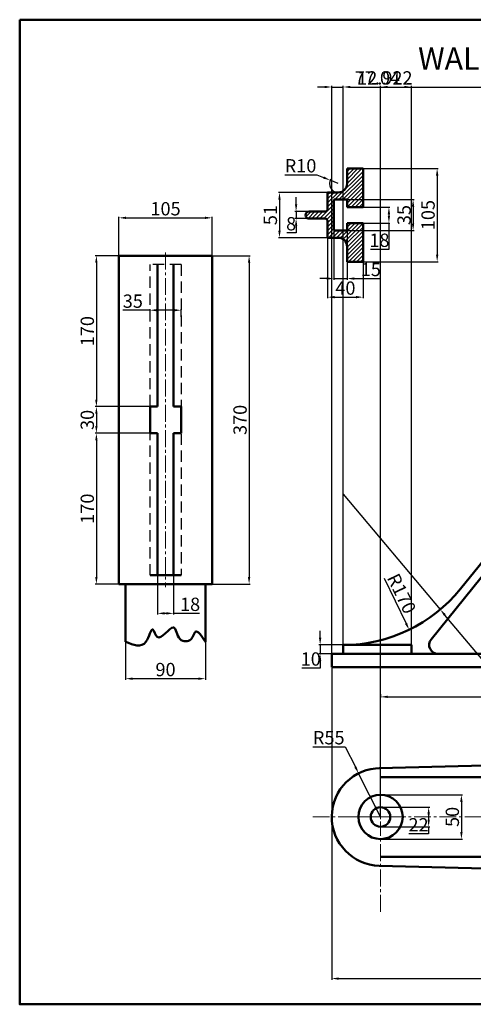
# Model space of a CAD drawing. Units: millimetres. Extents: x -60 to 1204, y -103 to 1006.
# Tile 1 of 4: x -60 to 452, y -103 to 1006. Entities that reach past the tile are written whole.
import ezdxf

# ---------------------------------------------------------------- set-up
doc = ezdxf.new("R2010")
doc.units = ezdxf.units.MM
doc.linetypes.add('CENTER2', pattern=[28.575, 19.05, -3.175, 3.175, -3.175])
doc.linetypes.add('DASHED', pattern=[19.05, 12.7, -6.35])
for name, color, linetype, lineweight in [('M-CNTR', 1, 'CENTER2', 18), ('M-DIMS', 2, 'Continuous', 25), ('M-HATC', 8, 'Continuous', 18), ('M-HIDN', 4, 'DASHED', 25), ('M-OUTL', 7, 'Continuous', 50), ('M-TEXT', 7, 'Continuous', 25), ('M-TTLB', 7, 'Continuous', 50)]:
    doc.layers.add(name, color=color, linetype=linetype, lineweight=lineweight)
doc.styles.get("Standard").update_dxf_attribs({"font": 'arial.ttf'})
doc.dimstyles.new('ISO-25', dxfattribs={"dimtxt": 15, "dimasz": 8, "dimexe": 1.25, "dimexo": 0.625, "dimtad": 1, "dimtoh": 1, "dimdec": 0, "dimtxsty": 'Standard', "dimcen": 2.5, "dimadec": 0, "dimazin": 0, "dimtfac": 1, "dimtdec": 0, "dimtmove": 0, "dimatfit": 3, "dimfxl": 1, "dimarcsym": 0})

# ---------------------------------------------------------------- blocks, each defined once
blk = doc.blocks.new('*U1')
at = {"layer": 'M-CNTR', "color": 0, "transparency": 16777216}
for p, q in [((0, 5), (0, 235.1)), ((-28.5, 0), (-5, 0)), ((5, 0), (28.5, 0)), ((0, -106.9), (0, -5))]:
    blk.add_line(p, q, dxfattribs=at)
at = {"layer": 'M-CNTR', "color": 0, "linetype": 'Continuous', "transparency": 16777216}
for p, q in [((-2.5, 0), (2.5, 0)), ((0, -2.5), (0, 2.5))]:
    blk.add_line(p, q, dxfattribs=at)
blk = doc.blocks.new('*U5')
at = {"layer": 'M-CNTR', "color": 0, "transparency": 16777216}
blk.add_line((0, 188.5), (0, -188.5), dxfattribs=at)
blk = doc.blocks.new('*D6')
at = {"layer": 'Defpoints', "color": 0, "transparency": 16777216}
for p in [(157.5, 740.2), (157.5, 370.2), (199.3, 370.2)]:
    blk.add_point(p, dxfattribs=at)
at = {"layer": 'M-DIMS', "color": 0, "lineweight": -2, "transparency": 16777216}
for p, q in [((158.1, 740.2), (200.5, 740.2)), ((199.3, 732.2), (199.3, 378.2)), ((158.1, 370.2), (200.5, 370.2))]:
    blk.add_line(p, q, dxfattribs=at)
at = {"layer": 'M-DIMS', "color": 0, "transparency": 16777216}
for points in [[(197.9, 732.2), (200.6, 732.2), (199.3, 740.2)], [(197.9, 378.2), (200.6, 378.2), (199.3, 370.2)]]:
    blk.add_solid(points, dxfattribs=at)
at = {"layer": 'M-DIMS', "color": 0, "transparency": 16777216, "insert": (191, 555.2), "char_height": 15, "attachment_point": 5, "rotation": 90}
blk.add_mtext('370', dxfattribs=at)
blk = doc.blocks.new('*D7')
at = {"layer": 'Defpoints', "color": 0, "transparency": 16777216}
for p in [(157.5, 782.9), (52.5, 740.2), (157.5, 740.2)]:
    blk.add_point(p, dxfattribs=at)
at = {"layer": 'M-DIMS', "color": 0, "lineweight": -2, "transparency": 16777216}
for p, q in [((52.5, 740.8), (52.5, 784.2)), ((60.5, 782.9), (149.5, 782.9)), ((157.5, 740.8), (157.5, 784.2))]:
    blk.add_line(p, q, dxfattribs=at)
at = {"layer": 'M-DIMS', "color": 0, "transparency": 16777216}
for points in [[(60.5, 784.2), (60.5, 781.6), (52.5, 782.9)], [(149.5, 784.2), (149.5, 781.6), (157.5, 782.9)]]:
    blk.add_solid(points, dxfattribs=at)
at = {"layer": 'M-DIMS', "color": 0, "transparency": 16777216, "insert": (105, 791.2), "char_height": 15, "attachment_point": 5}
blk.add_mtext('105', dxfattribs=at)
blk = doc.blocks.new('*D8')
at = {"layer": 'Defpoints', "color": 0, "transparency": 16777216}
for p in [(87.5, 570.2), (27, 540.2), (87.5, 540.2)]:
    blk.add_point(p, dxfattribs=at)
at = {"layer": 'M-DIMS', "color": 0, "lineweight": -2, "transparency": 16777216}
for p, q in [((86.9, 570.2), (25.7, 570.2)), ((27, 562.2), (27, 548.2)), ((86.9, 540.2), (25.7, 540.2))]:
    blk.add_line(p, q, dxfattribs=at)
at = {"layer": 'M-DIMS', "color": 0, "transparency": 16777216}
for points in [[(25.7, 562.2), (28.3, 562.2), (27, 570.2)], [(25.7, 548.2), (28.3, 548.2), (27, 540.2)]]:
    blk.add_solid(points, dxfattribs=at)
at = {"layer": 'M-DIMS', "color": 0, "transparency": 16777216, "insert": (18.7, 555.2), "char_height": 15, "attachment_point": 5, "rotation": 90}
blk.add_mtext('30', dxfattribs=at)
blk = doc.blocks.new('*D9')
at = {"layer": 'Defpoints', "color": 0, "transparency": 16777216}
for p in [(52.5, 740.2), (27, 570.2), (52.5, 570.2)]:
    blk.add_point(p, dxfattribs=at)
at = {"layer": 'M-DIMS', "color": 0, "lineweight": -2, "transparency": 16777216}
for p, q in [((51.9, 740.2), (25.7, 740.2)), ((27, 732.2), (27, 578.2)), ((51.9, 570.2), (25.7, 570.2))]:
    blk.add_line(p, q, dxfattribs=at)
at = {"layer": 'M-DIMS', "color": 0, "transparency": 16777216}
for points in [[(25.6, 732.2), (28.3, 732.2), (27, 740.2)], [(25.6, 578.2), (28.3, 578.2), (27, 570.2)]]:
    blk.add_solid(points, dxfattribs=at)
at = {"layer": 'M-DIMS', "color": 0, "transparency": 16777216, "insert": (18.7, 655.2), "char_height": 15, "attachment_point": 5, "rotation": 90}
blk.add_mtext('170', dxfattribs=at)
blk = doc.blocks.new('*D10')
at = {"layer": 'Defpoints', "color": 0, "transparency": 16777216}
for p in [(52.5, 540.2), (27, 370.2), (52.5, 370.2)]:
    blk.add_point(p, dxfattribs=at)
at = {"layer": 'M-DIMS', "color": 0, "lineweight": -2, "transparency": 16777216}
for p, q in [((51.9, 540.2), (25.7, 540.2)), ((27, 532.2), (27, 378.2)), ((51.9, 370.2), (25.7, 370.2))]:
    blk.add_line(p, q, dxfattribs=at)
at = {"layer": 'M-DIMS', "color": 0, "transparency": 16777216}
for points in [[(25.7, 532.2), (28.3, 532.2), (27, 540.2)], [(25.7, 378.2), (28.3, 378.2), (27, 370.2)]]:
    blk.add_solid(points, dxfattribs=at)
at = {"layer": 'M-DIMS', "color": 0, "transparency": 16777216, "insert": (18.7, 455.2), "char_height": 15, "attachment_point": 5, "rotation": 90}
blk.add_mtext('170', dxfattribs=at)
blk = doc.blocks.new('*D11')
at = {"layer": 'Defpoints', "color": 0, "transparency": 16777216}
for p in [(60, 321.7), (150, 321.7), (150, 263.7)]:
    blk.add_point(p, dxfattribs=at)
at = {"layer": 'M-DIMS', "color": 0, "lineweight": -2, "transparency": 16777216}
for p, q in [((60, 321.1), (60, 262.4)), ((150, 321.1), (150, 262.4)), ((68, 263.7), (142, 263.7))]:
    blk.add_line(p, q, dxfattribs=at)
at = {"layer": 'M-DIMS', "color": 0, "transparency": 16777216}
for points in [[(68, 265), (68, 262.3), (60, 263.7)], [(142, 265), (142, 262.3), (150, 263.7)]]:
    blk.add_solid(points, dxfattribs=at)
at = {"layer": 'M-DIMS', "color": 0, "transparency": 16777216, "insert": (105, 272), "char_height": 15, "attachment_point": 5}
blk.add_mtext('90', dxfattribs=at)
blk = doc.blocks.new('*D12')
at = {"layer": 'Defpoints', "color": 0, "transparency": 16777216}
for p in [(96, 380.2), (114, 380.2), (114, 337.3)]:
    blk.add_point(p, dxfattribs=at)
at = {"layer": 'M-DIMS', "color": 0, "lineweight": -2, "transparency": 16777216}
for p, q in [((96, 379.5), (96, 336)), ((114, 379.5), (114, 336)), ((104, 337.3), (106, 337.3)), ((114, 337.3), (143.4, 337.3))]:
    blk.add_line(p, q, dxfattribs=at)
at = {"layer": 'M-DIMS', "color": 0, "transparency": 16777216}
for points in [[(104, 338.6), (104, 335.9), (96, 337.3)], [(106, 338.6), (106, 335.9), (114, 337.3)]]:
    blk.add_solid(points, dxfattribs=at)
at = {"layer": 'M-DIMS', "color": 0, "transparency": 16777216, "insert": (132.7, 345.5), "char_height": 15, "attachment_point": 5}
blk.add_mtext('18', dxfattribs=at)
blk = doc.blocks.new('*D13')
at = {"layer": 'Defpoints', "color": 0, "transparency": 16777216}
for p in [(122.5, 678.8), (87.5, 670.6), (122.5, 670.6)]:
    blk.add_point(p, dxfattribs=at)
at = {"layer": 'M-DIMS', "color": 0, "lineweight": -2, "transparency": 16777216}
for p, q in [((87.5, 678.8), (56.7, 678.8)), ((87.5, 671.2), (87.5, 680.1)), ((114.5, 678.8), (95.5, 678.8)), ((122.5, 671.2), (122.5, 680.1))]:
    blk.add_line(p, q, dxfattribs=at)
at = {"layer": 'M-DIMS', "color": 0, "transparency": 16777216}
for points in [[(95.5, 680.2), (95.5, 677.5), (87.5, 678.8)], [(114.5, 680.2), (114.5, 677.5), (122.5, 678.8)]]:
    blk.add_solid(points, dxfattribs=at)
at = {"layer": 'M-DIMS', "color": 0, "transparency": 16777216, "insert": (68.1, 687.1), "char_height": 15, "attachment_point": 5}
blk.add_mtext('35', dxfattribs=at)
blk = doc.blocks.new('*D14')
at = {"layer": 'Defpoints', "color": 0, "transparency": 16777216}
for p in [(327.9, 795), (327.9, 777), (357, 777)]:
    blk.add_point(p, dxfattribs=at)
at = {"layer": 'M-DIMS', "color": 0, "lineweight": -2, "transparency": 16777216}
for p, q in [((328.5, 795), (358.2, 795)), ((328.5, 777), (358.2, 777)), ((357, 787), (357, 785)), ((357, 777), (357, 747.4)), ((357, 747.4), (336.3, 747.4))]:
    blk.add_line(p, q, dxfattribs=at)
at = {"layer": 'M-DIMS', "color": 0, "transparency": 16777216}
for points in [[(355.7, 787), (358.3, 787), (357, 795)], [(355.7, 785), (358.3, 785), (357, 777)]]:
    blk.add_solid(points, dxfattribs=at)
at = {"layer": 'M-DIMS', "color": 0, "transparency": 16777216, "insert": (346.3, 755.7), "char_height": 15, "attachment_point": 5}
blk.add_mtext('18', dxfattribs=at)
blk = doc.blocks.new('*D15')
at = {"layer": 'Defpoints', "color": 0, "transparency": 16777216}
for p in [(309.9, 803.5), (309.9, 768.5), (384.3, 768.5)]:
    blk.add_point(p, dxfattribs=at)
at = {"layer": 'M-DIMS', "color": 0, "lineweight": -2, "transparency": 16777216}
for p, q in [((310.5, 803.5), (385.5, 803.5)), ((384.3, 795.5), (384.3, 776.5)), ((310.5, 768.5), (385.5, 768.5))]:
    blk.add_line(p, q, dxfattribs=at)
at = {"layer": 'M-DIMS', "color": 0, "transparency": 16777216}
for points in [[(382.9, 795.5), (385.6, 795.5), (384.3, 803.5)], [(382.9, 776.5), (385.6, 776.5), (384.3, 768.5)]]:
    blk.add_solid(points, dxfattribs=at)
at = {"layer": 'M-DIMS', "color": 0, "transparency": 16777216, "insert": (376, 786), "char_height": 15, "attachment_point": 5, "rotation": 90}
blk.add_mtext('35', dxfattribs=at)
blk = doc.blocks.new('*D16')
at = {"layer": 'Defpoints', "color": 0, "transparency": 16777216}
for p in [(327.9, 838.5), (327.9, 733.5), (411.4, 733.5)]:
    blk.add_point(p, dxfattribs=at)
at = {"layer": 'M-DIMS', "color": 0, "lineweight": -2, "transparency": 16777216}
for p, q in [((328.5, 838.5), (412.7, 838.5)), ((411.4, 830.5), (411.4, 741.5)), ((328.5, 733.5), (412.7, 733.5))]:
    blk.add_line(p, q, dxfattribs=at)
at = {"layer": 'M-DIMS', "color": 0, "transparency": 16777216}
for points in [[(410.1, 830.5), (412.8, 830.5), (411.4, 838.5)], [(410.1, 741.5), (412.8, 741.5), (411.4, 733.5)]]:
    blk.add_solid(points, dxfattribs=at)
at = {"layer": 'M-DIMS', "color": 0, "transparency": 16777216, "insert": (403.1, 786), "char_height": 15, "attachment_point": 5, "rotation": 90}
blk.add_mtext('105', dxfattribs=at)
blk = doc.blocks.new('*D17')
at = {"layer": 'Defpoints', "color": 0, "transparency": 16777216}
for p in [(293.9, 811.5), (233.5, 760.5), (293.9, 760.5)]:
    blk.add_point(p, dxfattribs=at)
at = {"layer": 'M-DIMS', "color": 0, "lineweight": -2, "transparency": 16777216}
for p, q in [((293.2, 811.5), (232.3, 811.5)), ((233.5, 803.5), (233.5, 768.5)), ((293.2, 760.5), (232.3, 760.5))]:
    blk.add_line(p, q, dxfattribs=at)
at = {"layer": 'M-DIMS', "color": 0, "transparency": 16777216}
for points in [[(232.2, 803.5), (234.9, 803.5), (233.5, 811.5)], [(232.2, 768.5), (234.9, 768.5), (233.5, 760.5)]]:
    blk.add_solid(points, dxfattribs=at)
at = {"layer": 'M-DIMS', "color": 0, "transparency": 16777216, "insert": (225.2, 786), "char_height": 15, "attachment_point": 5, "rotation": 90}
blk.add_mtext('51', dxfattribs=at)
blk = doc.blocks.new('*D18')
at = {"layer": 'Defpoints', "color": 0, "transparency": 16777216}
for p in [(275.9, 790), (252.3, 782), (275.9, 782)]:
    blk.add_point(p, dxfattribs=at)
at = {"layer": 'M-DIMS', "color": 0, "lineweight": -2, "transparency": 16777216}
for p, q in [((252.3, 798), (252.3, 806)), ((275.2, 790), (251, 790)), ((252.3, 790), (252.3, 782)), ((275.2, 782), (251, 782)), ((252.3, 766), (241.8, 766)), ((252.3, 774), (252.3, 766))]:
    blk.add_line(p, q, dxfattribs=at)
at = {"layer": 'M-DIMS', "color": 0, "transparency": 16777216}
for points in [[(251, 798), (253.6, 798), (252.3, 790)], [(251, 774), (253.6, 774), (252.3, 782)]]:
    blk.add_solid(points, dxfattribs=at)
at = {"layer": 'M-DIMS', "color": 0, "transparency": 16777216, "insert": (246.7, 774.3), "char_height": 15, "attachment_point": 5}
blk.add_mtext('8', dxfattribs=at)
blk = doc.blocks.new('*D19')
at = {"layer": 'Defpoints', "color": 0, "transparency": 16777216}
for p in [(294.9, 768.5), (309.9, 768.5), (309.9, 714.5)]:
    blk.add_point(p, dxfattribs=at)
at = {"layer": 'M-DIMS', "color": 0, "lineweight": -2, "transparency": 16777216}
for p, q in [((294.9, 767.9), (294.9, 713.2)), ((309.9, 767.9), (309.9, 713.2)), ((286.9, 714.5), (278.9, 714.5)), ((294.9, 714.5), (309.9, 714.5)), ((317.9, 714.5), (347.3, 714.5))]:
    blk.add_line(p, q, dxfattribs=at)
at = {"layer": 'M-DIMS', "color": 0, "transparency": 16777216}
for points in [[(286.9, 715.8), (286.9, 713.1), (294.9, 714.5)], [(317.9, 715.8), (317.9, 713.1), (309.9, 714.5)]]:
    blk.add_solid(points, dxfattribs=at)
at = {"layer": 'M-DIMS', "color": 0, "transparency": 16777216, "insert": (336.6, 722.8), "char_height": 15, "attachment_point": 5}
blk.add_mtext('15', dxfattribs=at)
blk = doc.blocks.new('*D20')
at = {"layer": 'Defpoints', "color": 0, "transparency": 16777216}
for p in [(287.9, 760.5), (327.9, 733.5), (327.9, 693.5)]:
    blk.add_point(p, dxfattribs=at)
at = {"layer": 'M-DIMS', "color": 0, "lineweight": -2, "transparency": 16777216}
for p, q in [((287.9, 759.9), (287.9, 692.3)), ((327.9, 732.9), (327.9, 692.3)), ((295.9, 693.5), (319.9, 693.5))]:
    blk.add_line(p, q, dxfattribs=at)
at = {"layer": 'M-DIMS', "color": 0, "transparency": 16777216}
for points in [[(295.9, 694.9), (295.9, 692.2), (287.9, 693.5)], [(319.9, 694.9), (319.9, 692.2), (327.9, 693.5)]]:
    blk.add_solid(points, dxfattribs=at)
at = {"layer": 'M-DIMS', "color": 0, "transparency": 16777216, "insert": (307.9, 701.8), "char_height": 15, "attachment_point": 5}
blk.add_mtext('40', dxfattribs=at)
blk = doc.blocks.new('*D21')
at = {"layer": 'Defpoints', "color": 0, "transparency": 16777216}
for p in [(290.6, 825.3), (299.9, 821.5)]:
    blk.add_point(p, dxfattribs=at)
at = {"layer": 'M-DIMS', "color": 0, "lineweight": -2, "transparency": 16777216}
for p, q in [((239.4, 831.4), (275.8, 831.4)), ((275.8, 831.4), (283.2, 828.3)), ((299.9, 821.5), (290.6, 825.3))]:
    blk.add_line(p, q, dxfattribs=at)
blk.add_arc((299.9, 821.5), 10, 150.4971, 266.419, dxfattribs=at)
at = {"layer": 'M-DIMS', "color": 0, "transparency": 16777216}
blk.add_solid([(283.7, 829.6), (282.7, 827.1), (290.6, 825.3)], dxfattribs=at)
at = {"layer": 'M-DIMS', "color": 0, "transparency": 16777216, "insert": (257.3, 839.6), "char_height": 15, "attachment_point": 5}
blk.add_mtext('R10', dxfattribs=at)
blk = doc.blocks.new('*D49')
at = {"layer": 'Defpoints', "color": 0, "transparency": 16777216}
for p in [(305.5, 301.7), (279.4, 291.7), (305.5, 291.7)]:
    blk.add_point(p, dxfattribs=at)
at = {"layer": 'M-DIMS', "color": 0, "lineweight": -2, "transparency": 16777216}
for p, q in [((279.4, 309.7), (279.4, 317.7)), ((304.8, 301.7), (278.1, 301.7)), ((279.4, 301.7), (279.4, 291.7)), ((304.8, 291.7), (278.1, 291.7)), ((279.4, 283.7), (279.4, 275.7)), ((279.4, 275.7), (258.7, 275.7))]:
    blk.add_line(p, q, dxfattribs=at)
at = {"layer": 'M-DIMS', "color": 0, "transparency": 16777216}
for points in [[(278.1, 309.7), (280.7, 309.7), (279.4, 301.7)], [(278.1, 283.7), (280.7, 283.7), (279.4, 291.7)]]:
    blk.add_solid(points, dxfattribs=at)
at = {"layer": 'M-DIMS', "color": 0, "transparency": 16777216, "insert": (268.8, 283.9), "char_height": 15, "attachment_point": 5}
blk.add_mtext('10', dxfattribs=at)
blk = doc.blocks.new('*D50')
at = {"layer": 'Defpoints', "color": 0, "transparency": 16777216}
for p in [(305.5, 471.7), (379.8, 318.8)]:
    blk.add_point(p, dxfattribs=at)
at = {"layer": 'M-DIMS', "color": 0, "lineweight": -2, "transparency": 16777216}
blk.add_line((351.5, 377), (376.3, 326), dxfattribs=at)
at = {"layer": 'M-DIMS', "color": 0, "transparency": 16777216}
blk.add_solid([(377.5, 326.6), (375.1, 325.4), (379.8, 318.8)], dxfattribs=at)
at = {"layer": 'M-DIMS', "color": 0, "transparency": 16777216, "insert": (369.6, 358.7), "char_height": 15, "attachment_point": 5, "rotation": 295.9463}
blk.add_mtext('R170', dxfattribs=at)
blk = doc.blocks.new('*D51')
at = {"layer": 'Defpoints', "color": 0, "transparency": 16777216}
for p in [(347.5, 247), (947.5, 247), (947.5, 243.2)]:
    blk.add_point(p, dxfattribs=at)
at = {"layer": 'M-DIMS', "color": 0, "lineweight": -2, "transparency": 16777216}
for p, q in [((347.5, 246.4), (347.5, 242)), ((947.5, 246.4), (947.5, 242)), ((355.5, 243.2), (939.5, 243.2))]:
    blk.add_line(p, q, dxfattribs=at)
at = {"layer": 'M-DIMS', "color": 0, "transparency": 16777216}
for points in [[(355.5, 244.5), (355.5, 241.9), (347.5, 243.2)], [(939.5, 244.5), (939.5, 241.9), (947.5, 243.2)]]:
    blk.add_solid(points, dxfattribs=at)
at = {"layer": 'M-DIMS', "color": 0, "transparency": 16777216, "insert": (647.5, 251.5), "char_height": 15, "attachment_point": 5}
blk.add_mtext('600', dxfattribs=at)
blk = doc.blocks.new('*D57')
at = {"layer": 'Defpoints', "color": 0, "transparency": 16777216}
for p in [(347.5, 132.9), (347.5, 82.9), (438.8, 82.9)]:
    blk.add_point(p, dxfattribs=at)
at = {"layer": 'M-DIMS', "color": 0, "lineweight": -2, "transparency": 16777216}
for p, q in [((348.2, 132.9), (440, 132.9)), ((438.8, 124.9), (438.8, 90.9)), ((348.2, 82.9), (440, 82.9))]:
    blk.add_line(p, q, dxfattribs=at)
at = {"layer": 'M-DIMS', "color": 0, "transparency": 16777216}
for points in [[(437.4, 124.9), (440.1, 124.9), (438.8, 132.9)], [(437.4, 90.9), (440.1, 90.9), (438.8, 82.9)]]:
    blk.add_solid(points, dxfattribs=at)
at = {"layer": 'M-DIMS', "color": 0, "transparency": 16777216, "insert": (430.5, 107.9), "char_height": 15, "attachment_point": 5, "rotation": 90}
blk.add_mtext('50', dxfattribs=at)
blk = doc.blocks.new('*D58')
at = {"layer": 'Defpoints', "color": 0, "transparency": 16777216}
for p in [(347.5, 118.9), (347.5, 96.9), (401.8, 96.9)]:
    blk.add_point(p, dxfattribs=at)
at = {"layer": 'M-DIMS', "color": 0, "lineweight": -2, "transparency": 16777216}
for p, q in [((348.2, 118.9), (403.1, 118.9)), ((401.8, 110.9), (401.8, 104.9)), ((348.2, 96.9), (403.1, 96.9)), ((401.8, 88.9), (379.6, 88.9)), ((401.8, 96.9), (401.8, 88.9))]:
    blk.add_line(p, q, dxfattribs=at)
at = {"layer": 'M-DIMS', "color": 0, "transparency": 16777216}
for points in [[(400.5, 110.9), (403.2, 110.9), (401.8, 118.9)], [(400.5, 104.9), (403.2, 104.9), (401.8, 96.9)]]:
    blk.add_solid(points, dxfattribs=at)
at = {"layer": 'M-DIMS', "color": 0, "transparency": 16777216, "insert": (390.4, 97.1), "char_height": 15, "attachment_point": 5}
blk.add_mtext('22', dxfattribs=at)
blk = doc.blocks.new('*D59')
at = {"layer": 'Defpoints', "color": 0, "transparency": 16777216}
for p in [(322.8, 157), (347.5, 107.9)]:
    blk.add_point(p, dxfattribs=at)
at = {"layer": 'M-DIMS', "color": 0, "lineweight": -2, "transparency": 16777216}
for p, q in [((271.2, 187), (307.7, 187)), ((307.7, 187), (319.2, 164.2)), ((347.5, 107.9), (322.8, 157))]:
    blk.add_line(p, q, dxfattribs=at)
at = {"layer": 'M-DIMS', "color": 0, "transparency": 16777216}
blk.add_solid([(320.4, 164.8), (318, 163.6), (322.8, 157)], dxfattribs=at)
at = {"layer": 'M-DIMS', "color": 0, "transparency": 16777216, "insert": (289.1, 195.2), "char_height": 15, "attachment_point": 5}
blk.add_mtext('R55', dxfattribs=at)
blk = doc.blocks.new('*D61')
at = {"layer": 'Defpoints', "color": 0, "transparency": 16777216}
for p in [(292.5, 276.7), (1002.5, 276.7), (1002.5, -74.2)]:
    blk.add_point(p, dxfattribs=at)
at = {"layer": 'M-DIMS', "color": 0, "lineweight": -2, "transparency": 16777216}
for p, q in [((292.5, 276), (292.5, -75.5)), ((1002.5, 276), (1002.5, -75.5)), ((300.5, -74.2), (994.5, -74.2))]:
    blk.add_line(p, q, dxfattribs=at)
at = {"layer": 'M-DIMS', "color": 0, "transparency": 16777216}
for points in [[(300.5, -72.9), (300.5, -75.6), (292.5, -74.2)], [(994.5, -72.9), (994.5, -75.6), (1002.5, -74.2)]]:
    blk.add_solid(points, dxfattribs=at)
at = {"layer": 'M-DIMS', "color": 0, "transparency": 16777216, "insert": (647.5, -65.9), "char_height": 15, "attachment_point": 5}
blk.add_mtext('710', dxfattribs=at)
blk = doc.blocks.new('*D63')
at = {"layer": 'Defpoints', "color": 0, "transparency": 16777216}
for p in [(305.5, 930.3), (305.5, 301.7), (292.5, 291.7)]:
    blk.add_point(p, dxfattribs=at)
at = {"layer": 'M-DIMS', "color": 0, "lineweight": -2, "transparency": 16777216}
for p, q in [((284.5, 930.3), (276.5, 930.3)), ((292.5, 292.3), (292.5, 931.6)), ((292.5, 930.3), (305.5, 930.3)), ((305.5, 302.3), (305.5, 931.6)), ((313.5, 930.3), (383.4, 930.3))]:
    blk.add_line(p, q, dxfattribs=at)
at = {"layer": 'M-DIMS', "color": 0, "transparency": 16777216}
for points in [[(284.5, 931.6), (284.5, 929), (292.5, 930.3)], [(313.5, 931.6), (313.5, 929), (305.5, 930.3)]]:
    blk.add_solid(points, dxfattribs=at)
at = {"layer": 'M-DIMS', "color": 0, "transparency": 16777216, "insert": (352.4, 938.6), "char_height": 15, "attachment_point": 5}
blk.add_mtext('12.922', dxfattribs=at)
blk = doc.blocks.new('*D64')
at = {"layer": 'Defpoints', "color": 0, "transparency": 16777216}
for p in [(382.5, 930.3), (305.5, 301.7), (382.5, 301.7)]:
    blk.add_point(p, dxfattribs=at)
at = {"layer": 'M-DIMS', "color": 0, "lineweight": -2, "transparency": 16777216}
for p, q in [((305.5, 302.3), (305.5, 931.6)), ((313.5, 930.3), (374.5, 930.3)), ((382.5, 302.3), (382.5, 931.6))]:
    blk.add_line(p, q, dxfattribs=at)
at = {"layer": 'M-DIMS', "color": 0, "transparency": 16777216}
for points in [[(313.5, 931.6), (313.5, 929), (305.5, 930.3)], [(374.5, 931.6), (374.5, 929), (382.5, 930.3)]]:
    blk.add_solid(points, dxfattribs=at)
at = {"layer": 'M-DIMS', "color": 0, "transparency": 16777216, "insert": (344, 938.6), "char_height": 15, "attachment_point": 5}
blk.add_mtext('77.04', dxfattribs=at)
blk = doc.blocks.new('*D68')
at = {"layer": 'Defpoints', "color": 0, "transparency": 16777216}
for p in [(861.4, 930.3), (861.4, 175.8), (347.5, 107.9)]:
    blk.add_point(p, dxfattribs=at)
at = {"layer": 'M-DIMS', "color": 0, "lineweight": -2, "transparency": 16777216}
for p, q in [((347.5, 108.5), (347.5, 931.6)), ((355.5, 930.3), (853.4, 930.3)), ((861.4, 176.4), (861.4, 931.6))]:
    blk.add_line(p, q, dxfattribs=at)
at = {"layer": 'M-DIMS', "color": 0, "transparency": 16777216}
for points in [[(355.5, 931.6), (355.5, 929), (347.5, 930.3)], [(853.4, 931.6), (853.4, 929), (861.4, 930.3)]]:
    blk.add_solid(points, dxfattribs=at)
at = {"layer": 'M-DIMS', "color": 0, "transparency": 16777216, "insert": (604.5, 938.6), "char_height": 15, "attachment_point": 5}
blk.add_mtext('513.9', dxfattribs=at)
blk = doc.blocks.new('*D69')
at = {"layer": 'Defpoints', "color": 0, "transparency": 16777216}
for p in [(347.5, 152.9), (347.5, 62.9), (1144.5, 62.9)]:
    blk.add_point(p, dxfattribs=at)
at = {"layer": 'M-DIMS', "color": 0, "lineweight": -2, "transparency": 16777216}
for p, q in [((348.2, 152.9), (1145.7, 152.9)), ((1144.5, 144.9), (1144.5, 70.9)), ((348.2, 62.9), (1145.7, 62.9))]:
    blk.add_line(p, q, dxfattribs=at)
at = {"layer": 'M-DIMS', "color": 0, "transparency": 16777216}
for points in [[(1143.2, 144.9), (1145.8, 144.9), (1144.5, 152.9)], [(1143.2, 70.9), (1145.8, 70.9), (1144.5, 62.9)]]:
    blk.add_solid(points, dxfattribs=at)
at = {"layer": 'M-DIMS', "color": 0, "transparency": 16777216, "insert": (1136.2, 107.9), "char_height": 15, "attachment_point": 5, "rotation": 90}
blk.add_mtext('89.94', dxfattribs=at)
blk = doc.blocks.new('*D71')
at = {"layer": 'Defpoints', "color": 0, "transparency": 16777216}
for p in [(305.5, 471.7), (414.9, 341.6)]:
    blk.add_point(p, dxfattribs=at)
at = {"layer": 'M-DIMS', "color": 0, "lineweight": -2, "transparency": 16777216}
for p, q in [((305.5, 471.7), (414.9, 341.6)), ((480.5, 263.5), (420, 335.4)), ((528.6, 263.5), (480.5, 263.5))]:
    blk.add_line(p, q, dxfattribs=at)
at = {"layer": 'M-DIMS', "color": 0, "transparency": 16777216}
blk.add_solid([(421.1, 336.3), (419, 334.6), (414.9, 341.6)], dxfattribs=at)
at = {"layer": 'M-DIMS', "color": 0, "transparency": 16777216, "insert": (504.9, 271.8), "char_height": 15, "attachment_point": 5}
blk.add_mtext('R170', dxfattribs=at)

msp = doc.modelspace()

# ---------------------------------------------------------------- hatches: boundary and pattern name
at = {"layer": 'M-HATC'}
h = msp.add_hatch(dxfattribs=at)
h.set_pattern_fill('ANSI31', color=256)
h.paths.add_polyline_path([(327.8688, 838.4775), (309.8688, 838.4775), (309.8688, 821.4775, -0.414213562), (299.8688, 811.4775), (287.8688, 811.4775), (287.8688, 792.9775, -0.414213562), (284.8688, 789.9775), (266.8688, 789.9775, 1), (266.8688, 781.9775), (284.8688, 781.9775, -0.414213562), (287.8688, 778.9775), (287.8688, 760.4775), (299.8688, 760.4775, -0.414213562), (309.8688, 750.4775), (309.8688, 733.4775), (327.8688, 733.4775), (327.8688, 776.9775), (309.8688, 776.9775), (309.8688, 768.4775), (294.8688, 768.4775), (294.8688, 803.4775), (309.8688, 803.4775), (309.8688, 794.9775), (327.8688, 794.9775)])

# ---------------------------------------------------------------- linework, layer by layer
at = {"layer": 'M-CNTR'}
msp.add_line((271.0408, 107.9202), (1090.8372, 107.9202), dxfattribs=at)
at = {"layer": 'M-HIDN'}
for p, q in [((122.5027, 730.1606), (87.5027, 730.1606)), ((87.5027, 380.1606), (87.5027, 730.1606)), ((122.5027, 730.1606), (122.5027, 380.1606)), ((122.5027, 380.1606), (87.5027, 380.1606))]:
    msp.add_line(p, q, dxfattribs=at)
at = {"layer": 'M-OUTL', "ltscale": 0.5}
for p, q in [((437.7092, 364.8543), (828.5326, 848.7862)), ((404.6048, 307.9471), (831.6952, 836.7862)), ((305.4532, 301.6642), (347.5307, 301.6642))]:
    msp.add_line(p, q, dxfattribs=at)
at = {"layer": 'M-OUTL'}
for p, q in [((327.8688, 838.4775), (309.8688, 838.4775)), ((309.8688, 838.4775), (309.8688, 821.4775)), ((327.8688, 838.4775), (327.8688, 794.9775)), ((299.8688, 811.4775), (287.8688, 811.4775)), ((287.8688, 811.4775), (287.8688, 792.9775)), ((309.8688, 803.4775), (294.8688, 803.4775)), ((294.8688, 803.4775), (294.8688, 768.4775)), ((309.8688, 794.9775), (309.8688, 803.4775)), ((266.8688, 789.9775), (284.8688, 789.9775)), ((309.8688, 794.9775), (327.8688, 794.9775)), ((266.8688, 781.9775), (284.8688, 781.9775)), ((287.8688, 778.9775), (287.8688, 760.4775)), ((309.8688, 776.9775), (327.8688, 776.9775)), ((309.8688, 768.4775), (309.8688, 776.9775)), ((327.8688, 776.9775), (327.8688, 733.4775)), ((294.8688, 768.4775), (309.8688, 768.4775)), ((287.8688, 760.4775), (299.8688, 760.4775)), ((309.8688, 750.4775), (309.8688, 733.4775)), ((52.5027, 740.1606), (52.5027, 370.1606)), ((157.5027, 740.1606), (52.5027, 740.1606)), ((157.5027, 370.1606), (157.5027, 740.1606)), ((327.8688, 733.4775), (309.8688, 733.4775)), ((96.0027, 570.1606), (96.0027, 730.1606)), ((114.0027, 730.1606), (114.0027, 570.1606)), ((96.0027, 570.1606), (87.5027, 570.1606)), ((87.5027, 570.1606), (87.5027, 540.1606)), ((122.5027, 570.1606), (114.0027, 570.1606)), ((122.5027, 570.1606), (122.5027, 540.1606)), ((87.5027, 540.1606), (96.0027, 540.1606)), ((96.0027, 540.1606), (96.0027, 380.1606)), ((114.0027, 540.1606), (114.0027, 380.1606)), ((114.0027, 540.1606), (122.5027, 540.1606)), ((87.5027, 380.1606), (122.5027, 380.1606)), ((52.5027, 370.1606), (157.5027, 370.1606)), ((60.0027, 370.1606), (60.0027, 305.3374)), ((150.0027, 370.1606), (150.0027, 305.3374)), ((305.4532, 301.6642), (305.4532, 291.6642)), ((347.5307, 301.6642), (382.4937, 301.6642)), ((382.4937, 301.6642), (382.4937, 291.6642)), ((292.5307, 276.6642), (292.5307, 291.6642)), ((292.5307, 291.6642), (1002.5307, 291.6642)), ((292.5307, 276.6642), (1002.5307, 276.6642)), ((346.1577, 162.903), (861.3892, 175.7691)), ((700.8972, 152.892), (347.5307, 152.892)), ((700.8972, 62.9483), (347.5307, 62.9483)), ((346.1577, 52.9373), (861.3892, 40.0712))]:
    msp.add_line(p, q, dxfattribs=at)
for radius in [25, 11]:
    msp.add_circle((347.5307, 107.9202), radius, dxfattribs=at)
for centre, radius, start, end in [((299.8688, 821.4775), 10, 270, 0), ((266.8688, 785.9775), 4, 90, 270), ((284.8688, 792.9775), 3, 270, 0), ((284.8688, 778.9775), 3, 0, 90), ((299.8688, 750.4775), 10, 0, 90), ((412.3846, 301.6642), 10, 141.0756607, 270), ((347.5307, 107.9202), 55, 90, 268.5695401)]:
    msp.add_arc(centre, radius, start, end, dxfattribs=at)
at = {"layer": 'M-OUTL', "ltscale": 0.5}
msp.add_arc((305.4532, 471.6642), 170, 270, 321.0756607, dxfattribs=at)
at = {"layer": 'M-OUTL'}
msp.add_open_spline([(60.0027, 305.3374), (68.7895, 301.626), (83.591, 295.3742), (89.9116, 326.878), (96.2287, 300.2998), (116.2694, 332.976), (117.6565, 305.115), (135.1975, 304.9792), (138.5081, 322.6201), (145.5708, 312.0009), (150.0027, 305.3374)], degree=3, knots=[0, 0, 0, 0, 22.936069809, 38.635954019, 48.030377274, 69.245665278, 84.387647093, 96.840749142, 106.301605995, 122.239014618, 122.239014618, 122.239014618, 122.239014618], dxfattribs=at)
at = {"layer": 'M-TTLB'}
msp.add_lwpolyline([(-59.5454, 1006.1383), (1204.2342, 1006.1383), (1204.2342, -103.2116), (-59.5454, -103.2116)], close=True, dxfattribs=at)

# ---------------------------------------------------------------- block references
at = {"layer": 'M-CNTR'}
for name, p in [('*U5', (105.0027, 555.1606)), ('*U1', (347.5307, 107.9202))]:
    msp.add_blockref(name, p, dxfattribs=at)

# ---------------------------------------------------------------- texts
at = {"layer": 'M-TEXT', "insert": (389.9254, 974.8573), "char_height": 25, "attachment_point": 1}
msp.add_mtext_dynamic_manual_height_columns('WALL SUPPORT', width=382.720281, gutter_width=12.5, heights=[0], dxfattribs=at)

# ---------------------------------------------------------------- dimensions: what is measured, and where the dimension line sits
at = {"layer": 'M-DIMS'}
for base, p1, p2, override, picture, middle in [((305.45322, 930.31418), (292.53075, 291.66418), (305.45322, 301.66418), {"dimdec": 3, "dimlfac": 1, "dimrnd": 0, "dimzin": 0, "dimdsep": 46, "dimlunit": 2}, '*D63', (352.43122, 938.59778)), ((382.4937, 930.3142), (305.4532, 301.6642), (382.4937, 301.6642), {"dimdec": 2, "dimlfac": 1, "dimrnd": 0, "dimzin": 0, "dimdsep": 46, "dimlunit": 2}, '*D64', (343.9735, 938.5978)), ((861.3892, 930.3142), (347.5307, 107.9202), (861.3892, 175.7691), {"dimdec": 1, "dimlfac": 1, "dimrnd": 0, "dimzin": 0, "dimdsep": 46, "dimlunit": 2}, '*D68', (604.46, 938.6029)), ((157.5027, 782.911), (52.5027, 740.1606), (157.5027, 740.1606), {"dimclrd": 0, "dimclre": 0, "dimclrt": 0}, '*D7', (105.0027, 791.1946)), ((309.8688, 714.4685), (294.8688, 768.4775), (309.8688, 768.4775), {"dimclrd": 0, "dimclre": 0, "dimclrt": 0}, '*D19', (336.5876, 722.7521)), ((327.8688, 693.5264), (287.8688, 760.4775), (327.8688, 733.4775), {"dimclrd": 0, "dimclre": 0, "dimclrt": 0}, '*D20', (307.8688, 701.81)), ((114.0027, 337.2593), (96.0027, 380.1606), (114.0027, 380.1606), {"dimclrd": 0, "dimclre": 0, "dimclrt": 0}, '*D12', (132.6805, 345.5429)), ((150.0027, 263.6764), (60.0027, 321.6756), (150.0027, 321.6756), {"dimclrd": 0, "dimclre": 0, "dimclrt": 0}, '*D11', (105.0027, 271.96)), ((1002.5307, -74.2298), (292.5307, 276.6642), (1002.5307, 276.6642), {"dimdec": 0, "dimlfac": 1, "dimrnd": 0, "dimzin": 0, "dimdsep": 46, "dimlunit": 2}, '*D61', (647.5307, -65.9462)), ((947.5307, 243.2036), (347.5307, 246.9971), (947.5307, 246.9971), {"dimclrd": 0, "dimclre": 0, "dimclrt": 0}, '*D51', (647.5307, 251.4872))]:
    dim = msp.add_linear_dim(base=base, p1=p1, p2=p2, dimstyle='ISO-25', override=override, dxfattribs=at)
    dim.commit()
    dim.dimension.update_dxf_attribs({"geometry": picture, "text_midpoint": middle})
dim = msp.add_radius_dim(center=(299.8688, 821.4775), mpoint=(290.6194, 825.2787), dimstyle='ISO-25', override={"dimclrd": 0, "dimclre": 0, "dimclrt": 0}, dxfattribs=at)
dim.commit()
dim.dimension.update_dxf_attribs({"geometry": '*D21', "text_midpoint": (257.2998, 839.6442)})
for base, p1, p2, override, picture, middle in [((411.431, 733.4775), (327.8688, 838.4775), (327.8688, 733.4775), {"dimclrd": 0, "dimclre": 0, "dimclrt": 0}, '*D16', (403.1474, 785.9775)), ((233.5168, 760.4775), (293.8688, 811.4775), (293.8688, 760.4775), {"dimclrd": 0, "dimclre": 0, "dimclrt": 0}, '*D17', (225.2332, 785.9775)), ((252.2891, 781.9775), (275.8688, 789.9775), (275.8688, 781.9775), {"dimclrd": 0, "dimclre": 0, "dimclrt": 0}, '*D18', (246.7221, 774.2611)), ((384.2531, 768.4775), (309.8688, 803.4775), (309.8688, 768.4775), {"dimclrd": 0, "dimclre": 0, "dimclrt": 0}, '*D15', (375.9643, 785.9775)), ((26.9583, 570.1606), (52.5027, 740.1606), (52.5027, 570.1606), {"dimclrd": 0, "dimclre": 0, "dimclrt": 0}, '*D9', (18.6747, 655.1606)), ((199.2542, 370.1606), (157.5027, 740.1606), (157.5027, 370.1606), {"dimclrd": 0, "dimclre": 0, "dimclrt": 0}, '*D6', (190.9655, 555.1606)), ((26.9921, 540.1606), (87.5027, 570.1606), (87.5027, 540.1606), {"dimclrd": 0, "dimclre": 0, "dimclrt": 0}, '*D8', (18.7034, 555.1606)), ((26.9921, 370.1606), (52.5027, 540.1606), (52.5027, 370.1606), {"dimclrd": 0, "dimclre": 0, "dimclrt": 0}, '*D10', (18.7085, 455.1606)), ((279.3977, 291.6642), (305.4532, 301.6642), (305.4532, 291.6642), {"dimclrd": 0, "dimclre": 0, "dimclrt": 0}, '*D49', (268.7607, 283.9478)), ((1144.4872, 62.9483), (347.5307, 152.892), (347.5307, 62.9483), {"dimdec": 2, "dimlfac": 1, "dimrnd": 0, "dimzin": 0, "dimdsep": 46, "dimlunit": 2}, '*D69', (1136.2036, 107.9202)), ((438.7547, 82.9202), (347.5307, 132.9202), (347.5307, 82.9202), {"dimclrd": 0, "dimclre": 0, "dimclrt": 0}, '*D57', (430.4711, 107.9202)), ((401.8185, 96.9202), (347.5307, 118.9202), (347.5307, 96.9202), {"dimclrd": 0, "dimclre": 0, "dimclrt": 0}, '*D58', (390.3988, 97.0759))]:
    dim = msp.add_linear_dim(base=base, p1=p1, p2=p2, angle=90, dimstyle='ISO-25', override=override, dxfattribs=at)
    dim.commit()
    dim.dimension.update_dxf_attribs({"geometry": picture, "text_midpoint": middle})
dim = msp.add_linear_dim(base=(356.9915, 776.9775), p1=(327.8688, 794.9775), p2=(327.8688, 776.9775), angle=90, dimstyle='ISO-25', override={"dimclrd": 0, "dimclre": 0, "dimclrt": 0}, dxfattribs=at)
dim.commit()
dim.dimension.update_dxf_attribs({"geometry": '*D14', "text_midpoint": (346.3136, 747.3985), "dimtype": 160})
dim = msp.add_linear_dim(base=(122.5027, 678.8496), p1=(87.5027, 670.5609), p2=(122.5027, 670.5609), dimstyle='ISO-25', override={"dimclrd": 0, "dimclre": 0, "dimclrt": 0}, dxfattribs=at)
dim.commit()
dim.dimension.update_dxf_attribs({"geometry": '*D13', "text_midpoint": (68.083, 678.8496), "dimtype": 160})
for center, mpoint, override, picture, middle in [((305.4532, 471.6642), (379.8331, 318.7994), {"dimclrd": 0, "dimclre": 0, "dimclrt": 0}, '*D50', (362.1798, 355.0803)), ((305.4532, 471.6642), (414.8855, 341.5697), {"dimdec": 0, "dimlfac": 1, "dimrnd": 0, "dimzin": 0, "dimdsep": 46, "dimlunit": 2}, '*D71', (504.8926, 263.513)), ((347.5307, 107.9202), (322.797, 157.0449), {"dimclrd": 0, "dimclre": 0, "dimclrt": 0}, '*D59', (289.1329, 186.9592))]:
    dim = msp.add_radius_dim(center=center, mpoint=mpoint, dimstyle='ISO-25', override=override, dxfattribs=at)
    dim.commit()
    dim.dimension.update_dxf_attribs({"geometry": picture, "text_midpoint": middle, "dimtype": 164})

doc.saveas('drawing.dxf')
